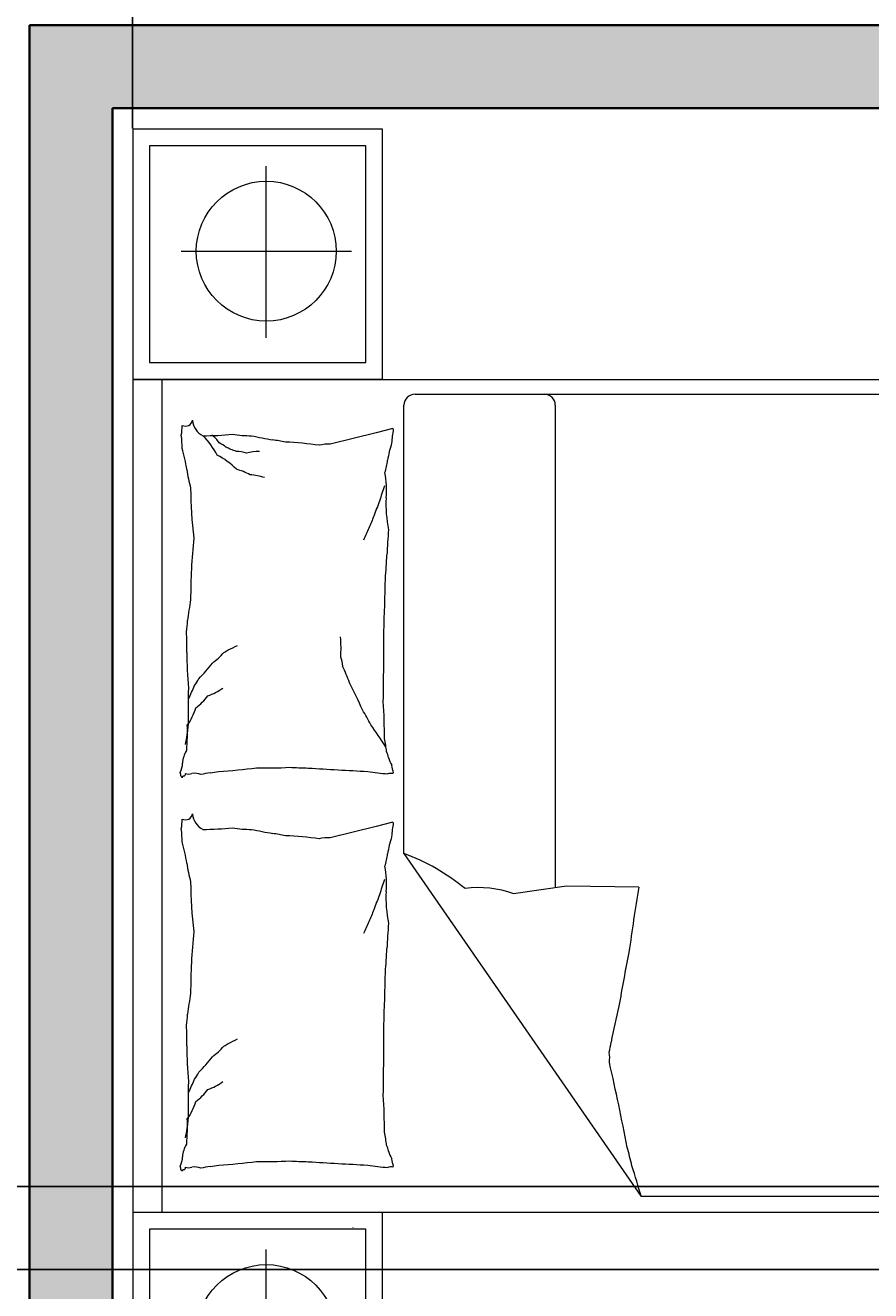
# Model space of a CAD drawing. Units: inches. Extents: x 2701 to 6846, y 811 to 2447.
# Tile 10 of 20: x 2780 to 2841, y 1371 to 1462. Entities that reach past the tile are written whole.
import ezdxf

# ---------------------------------------------------------------- set-up
doc = ezdxf.new("R2010")
doc.units = ezdxf.units.IN
for name, color, linetype, lineweight in [('A-ANNO-DIMS', 2, 'Continuous', 18), ('A-FLOR-PATT', 252, 'Continuous', 13), ('A-FURN', 8, 'Continuous', 13), ('A-WALL', 7, 'Continuous', 35)]:
    doc.layers.add(name, color=color, linetype=linetype, lineweight=lineweight)
doc.layers.add('A-WALL-PATT', color=18, linetype='Continuous', lineweight=13, true_color=0x000000)
doc.styles.add('DIM_FONT', font='SIMPLEX.shx', dxfattribs={"width": 0.8})
doc.styles.get("Standard").update_dxf_attribs({"font": 'arial.ttf'})
doc.dimstyles.get("Standard").update_dxf_attribs({"dimtxt": 0.18, "dimasz": 0.18, "dimexe": 0.18, "dimexo": 0.0625, "dimgap": 0.09, "dimtad": 0, "dimtih": 1, "dimtoh": 1, "dimdec": 4, "dimzin": 0, "dimdsep": 46, "dimtxsty": 'Standard', "dimcen": 0.09, "dimadec": 0, "dimazin": 0, "dimtfac": 1, "dimtdec": 4, "dimtofl": 0, "dimtmove": 0, "dimatfit": 3, "dimfxl": 1, "dimtolj": 1, "dimtzin": 0, "dimarcsym": 0})

# ---------------------------------------------------------------- blocks, each defined once
blk = doc.blocks.new('A$C187B6359')
for p, q in [((0.6993, 2.7052), (0.2493, 2.7052)), ((0.6993, 2.2552), (0.6993, 2.7052)), ((0.6999, 2.7053), (0.6999, 0.7053)), ((2.1999, 2.7053), (0.6999, 2.7053)), ((2.1999, 0.7053), (2.1999, 2.7053)), ((2.2013, 2.7052), (2.2013, 2.2552)), ((2.6513, 2.7052), (2.2013, 2.7052)), ((2.6513, 2.2552), (2.6513, 2.7052)), ((0.6693, 2.6752), (0.2793, 2.6752)), ((0.6693, 2.2852), (0.6693, 2.6752)), ((2.2313, 2.6752), (2.2313, 2.2852)), ((2.6213, 2.6752), (2.2313, 2.6752)), ((2.6213, 2.2852), (2.6213, 2.6752)), ((2.1999, 2.653), (0.6999, 2.653)), ((2.4317, 2.6178), (2.4317, 2.3115)), ((0.3236, 2.4648), (0.6327, 2.4648)), ((2.2756, 2.4648), (2.5847, 2.4648)), ((1.3953, 2.267), (1.3747, 2.3496)), ((2.1046, 2.267), (2.0839, 2.3496)), ((0.6727, 2.3088), (0.6721, 2.3088)), ((0.2793, 2.2852), (0.6693, 2.2852)), ((2.2313, 2.2852), (2.6213, 2.2852)), ((1.4029, 2.237), (1.3953, 2.267)), ((2.1121, 2.237), (2.1046, 2.267)), ((0.2493, 2.2552), (0.6993, 2.2552)), ((2.2013, 2.2552), (2.6513, 2.2552)), ((1.3464, 2.2168), (0.7284, 1.7894)), ((1.3464, 2.2168), (2.1541, 2.2168)), ((2.1741, 2.1968), (2.1741, 0.7375)), ((1.2876, 1.9238), (1.2739, 2.0192)), ((2.1541, 1.9442), (1.2846, 1.9442)), ((1.2858, 1.7936), (1.2876, 1.9238)), ((0.7284, 0.7375), (0.7284, 1.7894))]:
    blk.add_line(p, q)
for centre in [(0.4797, 2.4648), (2.4317, 2.4648)]:
    blk.add_circle(centre, 0.126)
for centre, radius, start, end in [((0.7725, 2.6193), 0.00342, 291.7883, 340.436), ((0.7743, 2.6138), 0.00232, 340.436, 101.8931), ((0.7738, 2.6432), 0.0251, 274.3025, 291.7883), ((0.7804, 2.6146), 0.00428, 201.9904, 281.8931), ((0.7958, 2.6048), 0.0156, 158.579, 201.9904), ((0.7979, 2.6447), 0.0289, 239.3487, 274.3025), ((0.7951, 2.5622), 0.0539, 59.3487, 84.7408), ((0.7953, 1.7882), 0.8208, 84.7408, 88.0921), ((0.8611, 2.7059), 0.0992, 254.0648, 274.2159), ((0.9268, 2.6871), 0.0992, 233.9136, 254.0648), ((0.8855, 1.1114), 1.4943, 88.0921, 90.5757), ((1.023, 2.8128), 0.234, 242.7604, 249.1397), ((1.0084, 1.7347), 0.8732, 90.5757, 94.8018), ((1.0124, 2.8973), 0.2897, 267.4614, 274.8018), ((1.0636, 2.7586), 0.1524, 259.8101, 267.4614), ((1.0008, 2.08), 0.5293, 79.8101, 83.9133), ((1.0944, 1.552), 1.049, 83.9133, 90), ((1.2953, 1.9183), 0.6827, 90, 97.5469), ((1.361, 2.3678), 0.2422, 97.5469, 105.744), ((1.2845, 2.9094), 0.3048, 278.4372, 285.744), ((1.3672, 2.7772), 0.1611, 270, 278.4372), ((1.4085, 2.7065), 0.0904, 258.7276, 270), ((1.4202, 2.6102), 0.0131, 153.4195, 258.7276), ((1.4817, 2.6193), 0.00342, 291.7883, 340.436), ((1.4835, 2.6138), 0.00232, 340.436, 101.8931), ((1.4831, 2.6432), 0.0251, 274.3025, 291.7883), ((1.4896, 2.6146), 0.00428, 201.9904, 281.8931), ((1.505, 2.6048), 0.0156, 158.579, 201.9904), ((1.5071, 2.6447), 0.0289, 239.3487, 274.3025), ((1.5043, 2.5622), 0.0539, 59.3487, 84.7408), ((1.5045, 1.7882), 0.8208, 84.7408, 88.0921), ((1.5703, 2.7059), 0.0992, 254.0648, 274.2159), ((1.6361, 2.6871), 0.0992, 233.9136, 254.0648), ((1.5948, 1.1114), 1.4943, 88.0921, 90.5757), ((1.7322, 2.8128), 0.234, 242.7604, 249.1397), ((1.7176, 1.7347), 0.8732, 90.5757, 94.8018), ((1.7217, 2.8973), 0.2897, 267.4614, 274.8018), ((1.7729, 2.7586), 0.1524, 259.8101, 267.4614), ((1.71, 2.08), 0.5293, 79.8101, 83.9133), ((1.8036, 1.552), 1.049, 83.9133, 90), ((2.0045, 1.9183), 0.6827, 90, 97.5469), ((2.0703, 2.3678), 0.2422, 97.5469, 105.744), ((1.9937, 2.9094), 0.3048, 278.4372, 285.744), ((2.0764, 2.7772), 0.1611, 270, 278.4372), ((2.1177, 2.7065), 0.0904, 258.7276, 270), ((2.1295, 2.6102), 0.0131, 153.4195, 258.7276), ((0.7489, 2.5943), 0.0328, 338.579, 8.1335), ((0.5389, 2.5307), 0.246, 8.1335, 12.1095), ((0.9797, 2.6502), 0.0992, 216.1766, 233.9136), ((0.9873, 2.6543), 0.0768, 231.6114, 242.7604), ((1.2233, 2.8687), 0.3916, 226.1885, 231.6114), ((1.4203, 2.5633), 0.0342, 94.4002, 153.4195), ((1.8817, 2.5789), 0.4918, 180, 186.2324), ((1.4581, 2.5943), 0.0328, 338.579, 8.1335), ((1.2481, 2.5307), 0.246, 8.1335, 12.1095), ((1.6889, 2.6502), 0.0992, 216.1766, 233.9136), ((1.6966, 2.6543), 0.0768, 231.6114, 242.7604), ((1.9325, 2.8687), 0.3916, 226.1885, 231.6114), ((2.0003, 2.6777), 0.1399, 297.2036, 314.9024), ((2.1295, 2.5633), 0.0342, 94.4002, 153.4195), ((2.5909, 2.5789), 0.4918, 180, 186.2324), ((0.979, 2.592), 0.1983, 187.6809, 192.1095), ((1.0154, 2.6015), 0.0992, 198.4397, 216.1766), ((1.155, 2.7035), 0.2252, 219.0349, 226.1885), ((1.6882, 2.592), 0.1983, 187.6809, 192.1095), ((1.7246, 2.6015), 0.0992, 198.4397, 216.1766), ((1.8643, 2.7035), 0.2252, 219.0349, 226.1885), ((2.0333, 2.622), 0.0899, 306.2641, 318.5571), ((1.6965, 2.6041), 0.9131, 183.3687, 187.6809), ((1.0425, 2.5644), 0.0493, 208.3168, 219.0349), ((1.1885, 2.6116), 0.2002, 203.0028, 208.3168), ((2.4058, 2.6041), 0.9131, 183.3687, 187.6809), ((1.7518, 2.5644), 0.0493, 208.3168, 219.0349), ((1.8977, 2.6116), 0.2002, 203.0028, 208.3168), ((1.9401, 2.6176), 0.1399, 314.9024, 332.6012), ((1.938, 2.5934), 0.1511, 334.6449, 338.1851), ((2.0389, 2.5721), 0.0526, 318.5571, 334.6449), ((1.5938, 2.4911), 0.204, 170.3156, 180), ((1.9047, 2.5583), 0.1399, 332.6012, 343.485), ((2.0146, 2.5185), 0.0562, 341.2201, 0), ((1.8799, 2.5949), 0.2056, 338.1851, 341.2201), ((2.3031, 2.4911), 0.204, 170.3156, 180), ((2.252, 2.3048), 0.882, 167.8016, 170.3156), ((1.8897, 2.5076), 0.1399, 343.485, 354.3689), ((1.9793, 2.4772), 0.0915, 0, 14.6851), ((2.9612, 2.3048), 0.882, 167.8016, 170.3156), ((1.4701, 2.4627), 0.6787, 178.3669, 183.3687), ((2.1793, 2.4627), 0.6787, 178.3669, 183.3687), ((1.0685, 2.4973), 0.3171, 347.8016, 351.9949), ((1.7777, 2.4973), 0.3171, 347.8016, 351.9949), ((2.1558, 2.35), 1.3652, 176.945, 178.3669), ((0.7204, 2.4609), 0.6588, 351.9949, 357.3351), ((2.8651, 2.35), 1.3652, 176.945, 178.3669), ((1.4296, 2.4609), 0.6588, 351.9949, 357.3351), ((14.4012, 1.5554), 13.6356, 176.49514, 176.94504), ((15.1105, 1.5554), 13.6356, 176.49514, 176.94504), ((1.3071, 2.3528), 0.0677, 357.3351, 14.0452), ((2.0163, 2.3528), 0.0677, 357.3351, 14.0452), ((1.4752, 2.7888), 0.5066, 290.6743, 294.3265), ((1.6798, 2.3849), 0.058, 274.0828, 290.6743), ((1.7172, 2.6022), 0.2721, 266.4448, 274.0828), ((1.0151, 3.5966), 1.4323, 294.3265, 296.4985), ((1.1013, 2.2263), 0.3212, 170.0016, 176.4951), ((0.9076, 1.6121), 0.7387, 64.6889, 66.5156), ((1.8106, 2.2263), 0.3212, 170.0016, 176.4951), ((1.4388, 2.5562), 0.3126, 296.4985, 302.135), ((1.6168, 1.6121), 0.7387, 64.6889, 66.5156), ((0.9508, 1.5933), 0.7387, 66.5156, 68.3423), ((0.9994, 1.5742), 0.7387, 68.3423, 70.572), ((1.0536, 1.5551), 0.7387, 70.572, 72.8018), ((1.1518, 2.8671), 0.7286, 302.135, 305.8263), ((1.66, 1.5933), 0.7387, 66.5156, 68.3423), ((1.7087, 1.5742), 0.7387, 68.3423, 70.572), ((1.7629, 1.5551), 0.7387, 70.572, 72.8018), ((0.7623, 2.2404), 0.0193, 350.0016, 16.6978), ((0.7815, 2.2357), 0.00132, 16.6978, 97.1204), ((0.8072, 2.1521), 0.0875, 97.1204, 106.2212), ((0.8315, 2.1707), 0.0767, 106.2212, 117.2841), ((0.8, 2.2885), 0.0453, 282.869, 297.2841), ((0.8116, 2.3939), 0.1459, 273.574, 282.869), ((0.8383, 3.4157), 1.164, 270.2865, 273.574), ((1.0077, 7.9716), 5.7185, 269.0296, 270.2865), ((1.1894, 5.6119), 3.3622, 267.3904, 269.0296), ((1.2304, 3.4627), 1.2165, 265.3824, 267.3904), ((1.1076, 0.8443), 1.4048, 85.3824, 87.2509), ((1.2668, 2.0191), 0.2301, 87.2509, 101.5586), ((1.2942, 2.3939), 0.1459, 263.5659, 281.5586), ((1.3592, 2.3652), 0.1197, 252.6136, 263.5659), ((1.3079, 2.0197), 0.2297, 72.6136, 80.5159), ((1.3573, 1.9688), 0.2708, 80.5159, 85.9171), ((1.4028, 2.2361), 0.000917, 85.9171, 194.0449), ((1.4715, 2.2404), 0.0193, 350.0016, 16.6978), ((1.4907, 2.2357), 0.00132, 16.6978, 97.1204), ((1.5164, 2.1521), 0.0875, 97.1204, 106.2212), ((1.5407, 2.1707), 0.0767, 106.2212, 117.2841), ((1.5092, 2.2885), 0.0453, 282.869, 297.2841), ((1.5209, 2.3939), 0.1459, 273.574, 282.869), ((1.5475, 3.4157), 1.164, 270.2865, 273.574), ((1.7169, 7.9716), 5.7185, 269.0296, 270.2865), ((1.8986, 5.6119), 3.3622, 267.3904, 269.0296), ((1.9396, 3.4627), 1.2165, 265.3824, 267.3904), ((1.8169, 0.8443), 1.4048, 85.3824, 87.2509), ((1.976, 2.0191), 0.2301, 87.2509, 101.5586), ((2.0034, 2.3939), 0.1459, 263.5659, 281.5586), ((2.0684, 2.3652), 0.1197, 252.6136, 263.5659), ((2.0172, 2.0197), 0.2297, 72.6136, 80.5159), ((2.0665, 1.9688), 0.2708, 80.5159, 85.9171), ((2.112, 2.2361), 0.000917, 85.9171, 194.0449), ((0.9943, 2.346), 0.3751, 320.3555, 339.8512), ((2.1541, 2.1968), 0.02, 0, 90), ((1.1048, 2.0812), 0.1801, 339.8512, 8.1356), ((2.1541, 1.9642), 0.02, 270, 0), ((0.9774, 1.9043), 0.0581, 262.2696, 280.7276), ((1.0326, 2.0362), 0.1942, 256.8096, 262.2696), ((0.0604, 5.8083), 4.0646, 280.7276, 282.9255), ((0.4974, -0.6199), 2.5158, 76.8096, 78.3259), ((0.6445, -0.723), 2.588, 78.3259, 80.505), ((0.2245, 3.554), 1.8351, 285.9352, 287.7364), ((0.6365, 2.4469), 0.6574, 282.9255, 285.9352), ((0.6623, -1.9346), 3.7801, 80.505, 82.308)]:
    blk.add_arc(centre, radius, start, end)
at = {"style": 'DIM_FONT', "text_generation_flag": 4, "width": 0.8, "flags": 9}
for tag in ['YSIZE', 'XSIZE']:
    blk.add_attdef(tag, (2.1999, 2.7053), '', height=0.0005, rotation=180, dxfattribs=at)
blk = doc.blocks.new('*D49')
at = {"layer": 'A-ANNO-DIMS', "color": 0, "lineweight": -2, "transparency": 16777216}
for p, q in [((2787.416, 1454.59), (2787.416, 1471.002)), ((2896.043, 1454.59), (2896.043, 1471.002)), ((2787.596, 1470.822), (2840.655, 1470.822)), ((2895.863, 1470.822), (2842.804, 1470.822))]:
    blk.add_line(p, q, dxfattribs=at)
at = {"layer": 'A-ANNO-DIMS', "color": 0, "transparency": 16777216}
for points in [[(2787.596, 1470.852), (2787.596, 1470.792), (2787.416, 1470.822)], [(2895.863, 1470.852), (2895.863, 1470.792), (2896.043, 1470.822)]]:
    blk.add_solid(points, dxfattribs=at)
at = {"layer": 'Defpoints', "color": 0, "transparency": 16777216}
for p in [(2787.416, 1470.822), (2787.416, 1454.528), (2896.043, 1454.528)]:
    blk.add_point(p, dxfattribs=at)
at = {"layer": 'A-ANNO-DIMS', "color": 0, "transparency": 16777216, "insert": (2841.729, 1470.822), "char_height": 0.18, "attachment_point": 5}
blk.add_mtext('\\A1;BED GROUP 109', dxfattribs=at)
blk = doc.blocks.new('*D75')
at = {"layer": 'A-ANNO-DIMS', "color": 0, "lineweight": -2, "transparency": 16777216}
for p, q in [((2923.909, 1378.05), (2700.591, 1378.05)), ((2700.771, 1377.87), (2700.771, 1375.232)), ((2700.771, 1372.23), (2700.771, 1374.868)), ((2923.909, 1372.05), (2700.591, 1372.05))]:
    blk.add_line(p, q, dxfattribs=at)
at = {"layer": 'A-ANNO-DIMS', "color": 0, "transparency": 16777216}
for points in [[(2700.741, 1377.87), (2700.801, 1377.87), (2700.771, 1378.05)], [(2700.741, 1372.23), (2700.801, 1372.23), (2700.771, 1372.05)]]:
    blk.add_solid(points, dxfattribs=at)
at = {"layer": 'Defpoints', "color": 0, "transparency": 16777216}
for p in [(2700.771, 1378.05), (2923.971, 1378.05), (2923.971, 1372.05)]:
    blk.add_point(p, dxfattribs=at)
at = {"layer": 'A-ANNO-DIMS', "color": 0, "transparency": 16777216, "insert": (2700.771, 1375.05), "char_height": 0.18, "attachment_point": 5}
blk.add_mtext('\\A1;6', dxfattribs=at)

msp = doc.modelspace()

# ---------------------------------------------------------------- hatches: boundary and pattern name
at = {"layer": 'A-FLOR-PATT'}
h = msp.add_hatch(dxfattribs=at)
h.set_pattern_fill('ANGLE', color=256)
h.set_pattern_definition([(0, (0, 0), (0, 6.985), [5.08, -1.905]), (90, (0, 0), (-6.985, 4e-16), [5.08, -1.905])])
h.paths.add_polyline_path([(2841.813, 1296.511, -0.109453), (2842.614, 1300.129, -0.102375), (2844.977, 1303.302, -0.093743), (2848.426, 1305.368, -0.062463), (2851.367, 1306.05), (2785.971, 1306.05), (2785.971, 1258.05), (2827.971, 1258.05), (2827.971, 1256.412), (2829.451, 1256.412, -0.394827), (2854.747, 1283.453), (2856.492, 1283.453), (2856.492, 1256.412), (2857.971, 1256.412), (2857.971, 1258.05), (2863.971, 1258.05), (2863.971, 1306.05), (2853.867, 1306.05, -0.062463), (2856.808, 1305.368, -0.093743), (2860.257, 1303.302, -0.102375), (2862.62, 1300.129, -0.109453), (2863.421, 1296.511, -0.109453), (2862.62, 1292.893, -0.102375), (2860.257, 1289.72, -0.093738), (2856.808, 1287.654, -0.088425), (2852.617, 1286.907, -0.088425), (2848.426, 1287.654, -0.093738), (2844.977, 1289.72, -0.102375), (2842.614, 1292.893, -0.109453)])
h.paths.add_polyline_path([(2805.215, 1273.877, -0.141745), (2808.319, 1271.773, -0.184983), (2809.774, 1267.974, -0.184983), (2808.319, 1264.176, -0.141745), (2805.215, 1262.071, -0.152244), (2799.994, 1261.796, -0.025614), (2799.369, 1261.945), (2794.365, 1263.418), (2794.365, 1263.405, -0.111242), (2793.993, 1261.915, -0.033889), (2793.114, 1260.114, -0.286745), (2792.376, 1259.652), (2787.581, 1259.652, -0.414214), (2787.153, 1260.08), (2787.153, 1267.974), (2787.153, 1275.869, -0.414214), (2787.581, 1276.297), (2792.376, 1276.297, -0.286745), (2793.114, 1275.835, -0.033889), (2793.993, 1274.033, -0.105104), (2794.362, 1272.628), (2794.365, 1272.53), (2799.369, 1274.003, -0.025614), (2799.994, 1274.153, -0.152244)], flags=16)
h.paths.add_polyline_path([(2804.681, 1272.34, -0.144945), (2807.088, 1270.709, -0.0358), (2807.447, 1270.253, -0.133285), (2807.893, 1268.608), (2807.893, 1267.974), (2807.893, 1267.341, -0.133285), (2807.447, 1265.696, -0.0358), (2807.088, 1265.24, -0.144945), (2804.681, 1263.609, -0.155404), (2800.343, 1263.386, -0.364511), (2796.485, 1267.974, -0.364511), (2800.343, 1272.563, -0.155404)], flags=0)
h.paths.add_polyline_path([(2800.016, 1268.901, 0.169298), (2799.131, 1268.116, 0.076667), (2799.1, 1267.974, 0.076667), (2799.131, 1267.833, 0.169298), (2800.016, 1267.047, 0.305219), (2800.365, 1267.156, 0.169535), (2800.651, 1267.974, 0.169535), (2800.365, 1268.792, 0.305219)], flags=0)
h.paths.add_polyline_path([(2971.971, 1456.05), (2923.971, 1456.05), (2923.971, 1408.05), (2922.333, 1408.05), (2922.333, 1406.571, -0.394827), (2949.374, 1381.274), (2949.374, 1379.529), (2922.333, 1379.529), (2922.333, 1378.05), (2923.971, 1378.05), (2923.971, 1372.05), (2971.971, 1372.05)])
h.paths.add_polyline_path([(2939.818, 1436.526, -0.141745), (2937.713, 1433.423, -0.184983), (2933.915, 1431.968, -0.184983), (2930.117, 1433.423, -0.141745), (2928.012, 1436.526, -0.152244), (2927.736, 1441.747, -0.025614), (2927.886, 1442.373), (2929.359, 1447.376), (2929.346, 1447.377, -0.111242), (2927.856, 1447.748, -0.033889), (2926.054, 1448.627, -0.286745), (2925.593, 1449.366), (2925.593, 1454.16, -0.414214), (2926.021, 1454.589), (2933.915, 1454.589), (2941.809, 1454.589, -0.414207), (2942.237, 1454.16), (2942.237, 1449.366, -0.286745), (2941.776, 1448.627, -0.033889), (2939.974, 1447.748, -0.105104), (2938.569, 1447.38), (2938.471, 1447.376), (2939.944, 1442.373, -0.025614), (2940.094, 1441.747, -0.152244)], flags=16)
h.paths.add_polyline_path([(2938.281, 1437.06, -0.144945), (2936.649, 1434.654, -0.0358), (2936.193, 1434.294, -0.133285), (2934.548, 1433.848), (2933.915, 1433.848), (2933.281, 1433.848, -0.133285), (2931.636, 1434.294, -0.0358), (2931.181, 1434.654, -0.144945), (2929.549, 1437.06, -0.155404), (2929.326, 1441.398, -0.364511), (2933.915, 1445.256, -0.364511), (2938.503, 1441.398, -0.155404)], flags=0)
h.paths.add_polyline_path([(2969.158, 1392.045, -0.093743), (2971.224, 1388.596, -0.088421), (2971.971, 1384.405, -0.088421), (2971.224, 1380.214, -0.093743), (2969.158, 1376.765, -0.102375), (2965.986, 1374.402, -0.109453), (2962.367, 1373.6, -0.109453), (2958.749, 1374.402, -0.102375), (2955.576, 1376.765, -0.093738), (2953.511, 1380.213, -0.088425), (2952.764, 1384.405, -0.088425), (2953.511, 1388.596, -0.093738), (2955.576, 1392.045, -0.102375), (2958.749, 1394.407, -0.109453), (2962.367, 1395.209, -0.109453), (2965.986, 1394.407, -0.102375)], flags=0)
edge = h.paths.add_edge_path(flags=16)
edge.add_arc((2961.075, 1384.859), 10.199, 20.2132, 41.63359, ccw=False)
edge.add_spline(control_points=[(2970.646, 1388.383), (2970.459, 1387.83), (2970.004, 1386.481), (2971.435, 1384.396), (2969.868, 1382.339), (2970.408, 1381.011), (2970.646, 1380.426)], knot_values=[0, 0, 0, 0, 0.041109, 0.100337, 0.155913, 0.199586, 0.199586, 0.199586, 0.199586], degree=3, periodic=0)
edge.add_arc((2961.075, 1383.95), 10.199, 318.36641, 339.7868, ccw=False)
edge.add_arc((2961.862, 1383.25), 9.145, 294.98529, 318.36641, ccw=False)
edge.add_arc((2962.367, 1382.166), 7.949, 269.99999, 294.98535, ccw=False)
edge.add_arc((2962.367, 1382.166), 7.949, 245.01465, 270.00002, ccw=False)
edge.add_arc((2962.873, 1383.25), 9.145, 221.63359, 245.01471, ccw=False)
edge.add_arc((2963.66, 1383.95), 10.199, 200.21296, 221.63359, ccw=False)
edge.add_arc((2964.894, 1384.405), 11.514, 180, 200.21296, ccw=False)
edge.add_arc((2964.894, 1384.405), 11.514, 159.78704, 179.99999, ccw=False)
edge.add_arc((2963.66, 1384.859), 10.199, 138.36641, 159.78704, ccw=False)
edge.add_arc((2962.873, 1385.559), 9.145, 114.98529, 138.36641, ccw=False)
edge.add_arc((2962.367, 1386.643), 7.949, 89.99999, 114.98534, ccw=False)
edge.add_arc((2962.367, 1386.643), 7.949, 65.01465, 90.00002, ccw=False)
edge.add_arc((2961.862, 1385.559), 9.145, 41.63359, 65.01471, ccw=False)
h.paths.add_polyline_path([(2963.81, 1393.327, -0.126458), (2966.613, 1390.683, -0.141697), (2967.169, 1388.761), (2967.169, 1387.406, -1), (2969.57, 1387.406, -0.414214), (2968.37, 1386.205), (2963.568, 1385.005, 0.146218), (2963.311, 1384.663), (2968.97, 1385.64), (2968.97, 1383.155), (2963.317, 1384.13, 0.140312), (2963.568, 1383.804), (2968.37, 1382.604, -0.414214), (2969.57, 1381.403, -1), (2967.169, 1381.403), (2967.169, 1380.04, -0.149025), (2966.557, 1378.032, -0.012759), (2966.265, 1377.619, -0.106303), (2963.81, 1375.482, -0.126822), (2961.167, 1374.801, -0.126822), (2958.524, 1375.482, -0.106303), (2956.069, 1377.619, -0.085722), (2954.537, 1380.623, -0.075351), (2953.964, 1384.405, -0.075351), (2954.537, 1388.187, -0.085722), (2956.069, 1391.19, -0.106303), (2958.524, 1393.327, -0.126822), (2961.167, 1394.009, -0.126822)], flags=0)
h.paths.add_polyline_path([(2934.842, 1441.725, 0.169298), (2934.056, 1442.61, 0.076667), (2933.915, 1442.641, 0.076667), (2933.773, 1442.61, 0.169298), (2932.988, 1441.725, 0.305219), (2933.097, 1441.376, 0.169535), (2933.915, 1441.09, 0.169535), (2934.733, 1441.376, 0.305219)], flags=0)
h.paths.add_polyline_path([(2969.324, 1387.406, -1), (2967.416, 1387.406, -1)], flags=0)
h.paths.add_polyline_path([(2968.831, 1387.406, -1), (2967.909, 1387.406, -1)], flags=0)
h.paths.add_polyline_path([(2962.13, 1384.357, -1), (2960.209, 1384.357, -1)], flags=0)
h.paths.add_polyline_path([(2961.801, 1384.357, -1), (2960.538, 1384.357, -1)], flags=0)
h.paths.add_polyline_path([(2969.324, 1381.403, -1), (2967.416, 1381.403, -1)], flags=0)
h.paths.add_polyline_path([(2968.831, 1381.403, -1), (2967.909, 1381.403, -1)], flags=0)
h.paths.add_polyline_path([(3085.971, 1306.05), (3001.971, 1306.05), (3001.971, 1300.05), (3000.333, 1300.05), (3000.333, 1298.571), (3027.374, 1298.571), (3027.374, 1296.826, -0.394827), (3000.333, 1271.529), (3000.333, 1270.05), (3001.971, 1270.05), (3001.971, 1258.05), (3085.971, 1258.05)])
h.paths.add_polyline_path([(3033.333, 1274.445, -0.102375), (3035.696, 1271.272, -0.109453), (3036.497, 1267.654, -0.109453), (3035.696, 1264.036, -0.102375), (3033.333, 1260.863, -0.093743), (3029.884, 1258.797, -0.088421), (3025.693, 1258.05, -0.088421), (3021.502, 1258.797, -0.093743), (3018.053, 1260.863, -0.102375), (3015.69, 1264.036, -0.109453), (3014.888, 1267.654, -0.109453), (3015.69, 1271.272, -0.102375), (3018.053, 1274.445, -0.093738), (3021.502, 1276.511, -0.088425), (3025.693, 1277.258, -0.088425), (3029.884, 1276.511, -0.093738)], flags=0)
edge = h.paths.add_edge_path(flags=16)
edge.add_arc((3026.847, 1267.149), 9.145, 24.98529, 48.36641, ccw=False)
edge.add_arc((3027.931, 1267.654), 7.949, -0.00001, 24.98534, ccw=False)
edge.add_arc((3027.931, 1267.654), 7.949, -24.98534, 0.00002, ccw=False)
edge.add_arc((3026.847, 1268.159), 9.145, 311.63359, 335.01471, ccw=False)
edge.add_arc((3026.147, 1268.947), 10.199, 290.2132, 311.63359, ccw=False)
edge.add_spline(control_points=[(3029.671, 1259.376), (3029.087, 1259.613), (3027.759, 1260.153), (3025.702, 1258.586), (3023.617, 1260.017), (3022.267, 1259.562), (3021.715, 1259.376)], knot_values=[0, 0, 0, 0, 0.043673, 0.099248, 0.158477, 0.199586, 0.199586, 0.199586, 0.199586], degree=3, periodic=0)
edge.add_arc((3025.239, 1268.947), 10.199, 228.36641, 249.7868, ccw=False)
edge.add_arc((3024.538, 1268.159), 9.145, 204.98529, 228.36641, ccw=False)
edge.add_arc((3023.454, 1267.654), 7.949, 179.99999, 204.98534, ccw=False)
edge.add_arc((3023.454, 1267.654), 7.949, 155.01465, 180.00002, ccw=False)
edge.add_arc((3024.538, 1267.149), 9.145, 131.63359, 155.01471, ccw=False)
edge.add_arc((3025.239, 1266.361), 10.199, 110.21296, 131.63359, ccw=False)
edge.add_arc((3025.693, 1265.127), 11.514, 90, 110.21296, ccw=False)
edge.add_arc((3025.693, 1265.127), 11.514, 69.78704, 89.99999, ccw=False)
edge.add_arc((3026.147, 1266.361), 10.199, 48.36641, 69.78704, ccw=False)
h.paths.add_polyline_path([(3032.478, 1273.952, -0.106303), (3034.615, 1271.497, -0.126822), (3035.297, 1268.854, -0.126822), (3034.615, 1266.212, -0.106303), (3032.478, 1263.757, -0.012759), (3032.066, 1263.464, -0.149025), (3030.057, 1262.852), (3028.694, 1262.852, -0.414214), (3029.895, 1261.652, -1), (3027.494, 1261.652), (3026.293, 1266.453, 0.140312), (3025.968, 1266.704), (3026.943, 1261.051), (3024.458, 1261.051), (3025.434, 1266.71, 0.146218), (3025.093, 1266.453), (3023.892, 1261.652, -1), (3021.491, 1261.652, -0.414214), (3022.692, 1262.852), (3021.337, 1262.852, -0.141697), (3019.415, 1263.408, -0.126458), (3016.77, 1266.212, -0.126822), (3016.089, 1268.854, -0.126822), (3016.77, 1271.497, -0.106303), (3018.908, 1273.952, -0.085722), (3021.911, 1275.484, -0.075351), (3025.693, 1276.057, -0.075351), (3029.475, 1275.484, -0.085722)], flags=0)
h.paths.add_polyline_path([(3072.365, 1280.002, -0.184983), (3076.163, 1281.457, -0.184983), (3079.961, 1280.002, -0.141745), (3082.066, 1276.898, -0.152244), (3082.342, 1271.678, -0.025614), (3082.192, 1271.052), (3080.719, 1266.048), (3080.817, 1266.045, -0.105104), (3082.222, 1265.676, -0.033889), (3084.024, 1264.798, -0.286745), (3084.485, 1264.059), (3084.485, 1259.264, -0.41422), (3084.057, 1258.836), (3076.163, 1258.836), (3068.269, 1258.836, -0.414214), (3067.841, 1259.264), (3067.841, 1264.059, -0.286745), (3068.302, 1264.798, -0.033889), (3070.104, 1265.676, -0.105104), (3071.509, 1266.045), (3071.607, 1266.048), (3070.134, 1271.052, -0.025614), (3069.984, 1271.678, -0.152244), (3070.26, 1276.898, -0.141745)], flags=16)
h.paths.add_polyline_path([(3073.429, 1278.771, -0.0358), (3073.885, 1279.13, -0.133285), (3075.529, 1279.577), (3076.163, 1279.577), (3076.797, 1279.577, -0.133285), (3078.441, 1279.13, -0.0358), (3078.897, 1278.771, -0.144945), (3080.529, 1276.364, -0.155404), (3080.752, 1272.026, -0.364511), (3076.163, 1268.168, -0.364511), (3071.574, 1272.026, -0.155404), (3071.797, 1276.364, -0.144945)], flags=0)
h.paths.add_polyline_path([(3026.7, 1268.852, -1), (3024.78, 1268.852, -1)], flags=0)
h.paths.add_polyline_path([(3026.372, 1268.852, -1), (3025.108, 1268.852, -1)], flags=0)
h.paths.add_polyline_path([(3075.269, 1271.624, 0.157677), (3076.022, 1270.814, 0.076667), (3076.163, 1270.783, 0.076667), (3076.304, 1270.814, 0.157677), (3077.058, 1271.624, 0.374626), (3076.981, 1272.048, 0.169535), (3076.163, 1272.334, 0.169535), (3075.345, 1272.048, 0.374626)], flags=0)
h.paths.add_polyline_path([(3029.648, 1261.652, -1), (3027.74, 1261.652, -1)], flags=0)
h.paths.add_polyline_path([(3029.155, 1261.652, -1), (3028.233, 1261.652, -1)], flags=0)
h.paths.add_polyline_path([(3023.646, 1261.652, -1), (3021.738, 1261.652, -1)], flags=0)
h.paths.add_polyline_path([(3023.152, 1261.652, -1), (3022.231, 1261.652, -1)], flags=0)
h.paths.add_polyline_path([(2810.573, 1281.222), (2833.311, 1281.222), (2833.311, 1296.429), (2810.573, 1296.429)], flags=24)
h.paths.add_polyline_path([(2937.545, 1410.244), (2960.208, 1410.244), (2960.208, 1425.452), (2937.545, 1425.452)], flags=24)
h.paths.add_polyline_path([(3043.228, 1273.099), (3065.891, 1273.099), (3065.891, 1288.306), (3043.228, 1288.306)], flags=24)
at = {"layer": 'A-WALL-PATT'}
h = msp.add_hatch(color=256, dxfattribs=at)
h.dxf.hatch_style = 1
h.paths.add_polyline_path([(3085.971, 1456.05), (3085.971, 1348.05), (3091.971, 1348.05), (3091.971, 1360.05), (3091.971, 1462.05), (2960.086, 1462.05), (2960.086, 1456.05), (2971.971, 1456.05), (2971.971, 1372.05), (2923.971, 1372.05), (2923.971, 1378.05), (2917.971, 1378.05), (2917.971, 1351.05), (2923.971, 1351.05), (2923.971, 1366.05), (2971.971, 1366.05), (2971.971, 1351.05), (2976.769, 1351.05), (2977.971, 1351.05), (2977.971, 1456.05)])
h.paths.add_polyline_path([(2779.971, 1462.05), (2779.971, 1342.05), (2785.971, 1342.05), (2785.971, 1456.05), (2917.971, 1456.05), (2917.971, 1408.05), (2922.333, 1408.05), (2923.971, 1408.05), (2923.971, 1456.05), (2937.086, 1456.05), (2937.086, 1462.05)])
h.paths.add_polyline_path([(2779.971, 1306.05), (2779.971, 1294.241), (2785.971, 1294.241), (2785.971, 1306.05), (2851.367, 1306.05, -0.025815), (2852.617, 1306.115, -0.025815), (2853.867, 1306.05), (2863.971, 1306.05), (2863.971, 1258.05), (2857.971, 1258.05), (2857.971, 1252.05), (2878.971, 1252.05), (2878.971, 1258.05), (2869.971, 1258.05), (2869.971, 1306.05), (2923.971, 1306.05), (2923.971, 1318.05), (2919.174, 1318.05), (2917.971, 1318.05), (2917.971, 1312.05), (2785.971, 1312.05), (2785.971, 1318.05), (2779.971, 1318.05)])
h.paths.add_polyline_path([(2785.971, 1252.05), (2827.971, 1252.05), (2827.971, 1256.412), (2827.971, 1258.05), (2785.971, 1258.05), (2785.971, 1271.241), (2779.971, 1271.241), (2779.971, 1174.05), (2785.971, 1174.05)])
h.paths.add_polyline_path([(2779.971, 1030.05), (2869.971, 1030.05), (2869.971, 1036.05), (2785.971, 1036.05), (2785.971, 1126.05), (2917.971, 1126.05), (2917.971, 1120.05), (2923.971, 1120.05), (2923.971, 1258.05), (2911.971, 1258.05), (2911.971, 1253.252), (2911.971, 1252.05), (2917.971, 1252.05), (2917.971, 1132.05), (2785.971, 1132.05), (2785.971, 1144.05), (2779.971, 1144.05)])
h.paths.add_polyline_path([(2935.971, 1030.05), (2935.971, 1033.05), (2935.971, 1036.05), (2923.971, 1036.05), (2923.971, 1087.05), (2919.174, 1087.05), (2917.971, 1087.05), (2917.971, 1036.05), (2893.971, 1036.05), (2893.971, 1030.05)])
h.paths.add_polyline_path([(2971.971, 1036.05), (2971.971, 1030.05), (3091.971, 1030.05), (3091.971, 1060.05), (3085.971, 1060.05), (3085.971, 1036.05)])
h.paths.add_polyline_path([(3085.971, 1084.05), (3091.971, 1084.05), (3091.971, 1096.05), (3091.971, 1268.891), (3085.971, 1268.891), (3085.971, 1258.05), (3001.971, 1258.05), (3001.971, 1270.05), (2995.971, 1270.05), (2995.971, 1252.05), (3085.971, 1252.05)])
h.paths.add_polyline_path([(3085.971, 1306.05), (3085.971, 1291.891), (3091.971, 1291.891), (3091.971, 1318.05), (3085.971, 1318.05), (3085.971, 1312.05), (2977.971, 1312.05), (2977.971, 1318.05), (2971.971, 1318.05), (2971.971, 1306.05), (2995.971, 1306.05), (2995.971, 1300.05), (3000.333, 1300.05), (3001.971, 1300.05), (3001.971, 1306.05)])

# ---------------------------------------------------------------- linework, layer by layer
at = {"layer": 'A-WALL'}
for p, q in [((3091.971, 1462.05), (2779.971, 1462.05)), ((2779.971, 1030.05), (2779.971, 1462.05)), ((2785.971, 1312.05), (2785.971, 1456.05)), ((2917.971, 1456.05), (2785.971, 1456.05))]:
    msp.add_line(p, q, dxfattribs=at)

# ---------------------------------------------------------------- block references
at = {"layer": 'A-FURN', "xscale": 40.14518915969158, "yscale": 40.14518915969158, "zscale": 40.14518915969158, "rotation": 90}
msp.add_blockref('A$C187B6359', (2896.043, 1348.092), dxfattribs=at)

# ---------------------------------------------------------------- dimensions: what is measured, and where the dimension line sits
at = {"layer": 'A-ANNO-DIMS'}
dim = msp.add_linear_dim(base=(2787.416, 1470.822), p1=(2896.043, 1454.528), p2=(2787.416, 1454.528), angle=180, text='BED GROUP <>', dimstyle='Standard', override={"dimdec": 0, "dimlfac": 1, "dimrnd": 0, "dimzin": 0, "dimdsep": 46, "dimlunit": 2}, dxfattribs=at)
dim.commit()
dim.dimension.update_dxf_attribs({"geometry": '*D49', "text_midpoint": (2841.729, 1470.822)})
dim = msp.add_linear_dim(base=(2700.771, 1378.05), p1=(2923.971, 1372.05), p2=(2923.971, 1378.05), angle=90, dimstyle='Standard', override={"dimdec": 0, "dimlfac": 1, "dimrnd": 0, "dimzin": 0, "dimdsep": 46, "dimlunit": 2}, dxfattribs=at)
dim.commit()
dim.dimension.update_dxf_attribs({"geometry": '*D75', "text_midpoint": (2700.771, 1375.05)})

doc.saveas('drawing.dxf')
